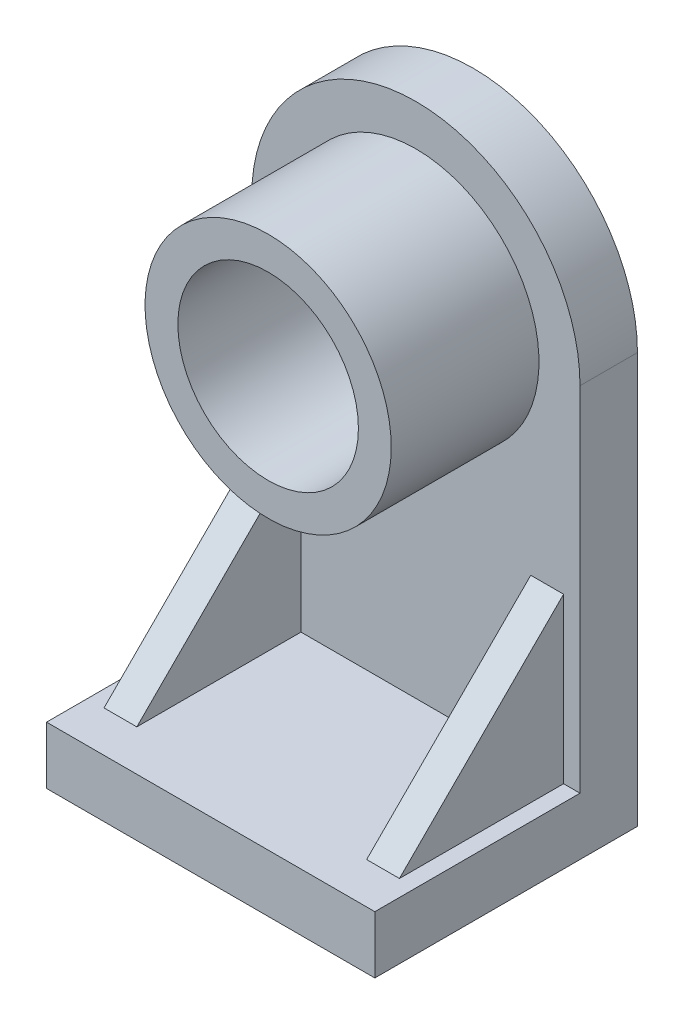
ISO-10303-21;
HEADER;
FILE_DESCRIPTION(('STEP AP214'),'2;1');
FILE_NAME('part.step','',(''),(''),'','','');
FILE_SCHEMA(('AUTOMOTIVE_DESIGN { 1 0 10303 214 1 1 1 1 }'));
ENDSEC;
DATA;
#1=APPLICATION_CONTEXT('core data for automotive mechanical design processes');
#2=APPLICATION_PROTOCOL_DEFINITION('international standard','automotive_design',2000,#1);
#3=PRODUCT_CONTEXT('',#1,'mechanical');
#4=PRODUCT('Part','Part','',(#3));
#5=PRODUCT_RELATED_PRODUCT_CATEGORY('part','',(#4));
#6=PRODUCT_DEFINITION_FORMATION('','',#4);
#7=PRODUCT_DEFINITION_CONTEXT('part definition',#1,'design');
#8=PRODUCT_DEFINITION('design','',#6,#7);
#9=PRODUCT_DEFINITION_SHAPE('','',#8);
#10=(LENGTH_UNIT() NAMED_UNIT(*) SI_UNIT(.MILLI.,.METRE.));
#11=(NAMED_UNIT(*) PLANE_ANGLE_UNIT() SI_UNIT($,.RADIAN.));
#12=(NAMED_UNIT(*) SI_UNIT($,.STERADIAN.) SOLID_ANGLE_UNIT());
#13=UNCERTAINTY_MEASURE_WITH_UNIT(LENGTH_MEASURE(1.E-05),#10,'distance_accuracy_value','');
#14=(GEOMETRIC_REPRESENTATION_CONTEXT(3) GLOBAL_UNCERTAINTY_ASSIGNED_CONTEXT((#13)) GLOBAL_UNIT_ASSIGNED_CONTEXT((#10,
#11,#12)) REPRESENTATION_CONTEXT('',''));
#15=CARTESIAN_POINT('',(0.,0.,0.));
#16=DIRECTION('',(0.,0.,1.));
#17=DIRECTION('',(1.,0.,0.));
#18=AXIS2_PLACEMENT_3D('',#15,#16,#17);
#19=CARTESIAN_POINT('',(20.,7.,0.));
#20=DIRECTION('',(0.,0.,-1.));
#21=DIRECTION('',(0.,1.,0.));
#22=AXIS2_PLACEMENT_3D('',#19,#20,#21);
#23=PLANE('',#22);
#24=DIRECTION('',(0.,-1.,0.));
#25=VECTOR('',#24,1.);
#26=CARTESIAN_POINT('',(-20.,7.,0.));
#27=LINE('',#26,#25);
#28=CARTESIAN_POINT('',(-20.,7.,0.));
#29=VERTEX_POINT('',#28);
#30=CARTESIAN_POINT('',(-20.,0.,0.));
#31=VERTEX_POINT('',#30);
#32=EDGE_CURVE('E189',#29,#31,#27,.T.);
#33=ORIENTED_EDGE('',*,*,#32,.T.);
#34=DIRECTION('',(-1.,0.,0.));
#35=VECTOR('',#34,1.);
#36=CARTESIAN_POINT('',(20.,0.,0.));
#37=LINE('',#36,#35);
#38=CARTESIAN_POINT('',(20.,0.,0.));
#39=VERTEX_POINT('',#38);
#40=EDGE_CURVE('E48',#39,#31,#37,.T.);
#41=ORIENTED_EDGE('',*,*,#40,.F.);
#42=DIRECTION('',(0.,-1.,0.));
#43=VECTOR('',#42,1.);
#44=CARTESIAN_POINT('',(20.,7.,0.));
#45=LINE('',#44,#43);
#46=CARTESIAN_POINT('',(20.,7.,0.));
#47=VERTEX_POINT('',#46);
#48=EDGE_CURVE('E195',#47,#39,#45,.T.);
#49=ORIENTED_EDGE('',*,*,#48,.F.);
#50=DIRECTION('',(-1.,0.,0.));
#51=VECTOR('',#50,1.);
#52=CARTESIAN_POINT('',(20.,7.,0.));
#53=LINE('',#52,#51);
#54=EDGE_CURVE('E206',#47,#29,#53,.T.);
#55=ORIENTED_EDGE('',*,*,#54,.T.);
#56=EDGE_LOOP('',(#33,#41,#49,#55));
#57=FACE_BOUND('',#56,.T.);
#58=ADVANCED_FACE('F41',(#57),#23,.F.);
#59=CARTESIAN_POINT('',(20.,0.,0.));
#60=DIRECTION('',(0.,1.,0.));
#61=DIRECTION('',(0.,0.,1.));
#62=AXIS2_PLACEMENT_3D('',#59,#60,#61);
#63=PLANE('',#62);
#64=DIRECTION('',(0.,0.,-1.));
#65=VECTOR('',#64,1.);
#66=CARTESIAN_POINT('',(-20.,0.,0.));
#67=LINE('',#66,#65);
#68=CARTESIAN_POINT('',(-20.,0.,-32.));
#69=VERTEX_POINT('',#68);
#70=EDGE_CURVE('E207',#31,#69,#67,.T.);
#71=ORIENTED_EDGE('',*,*,#70,.T.);
#72=DIRECTION('',(-1.,0.,0.));
#73=VECTOR('',#72,1.);
#74=CARTESIAN_POINT('',(20.,0.,-32.));
#75=LINE('',#74,#73);
#76=CARTESIAN_POINT('',(20.,0.,-32.));
#77=VERTEX_POINT('',#76);
#78=EDGE_CURVE('E224',#77,#69,#75,.T.);
#79=ORIENTED_EDGE('',*,*,#78,.F.);
#80=DIRECTION('',(0.,0.,-1.));
#81=VECTOR('',#80,1.);
#82=CARTESIAN_POINT('',(20.,0.,0.));
#83=LINE('',#82,#81);
#84=EDGE_CURVE('E194',#39,#77,#83,.T.);
#85=ORIENTED_EDGE('',*,*,#84,.F.);
#86=ORIENTED_EDGE('',*,*,#40,.T.);
#87=EDGE_LOOP('',(#71,#79,#85,#86));
#88=FACE_BOUND('',#87,.T.);
#89=ADVANCED_FACE('F226',(#88),#63,.F.);
#90=CARTESIAN_POINT('',(20.,0.,-32.));
#91=DIRECTION('',(0.,0.,1.));
#92=DIRECTION('',(0.,-1.,0.));
#93=AXIS2_PLACEMENT_3D('',#90,#91,#92);
#94=PLANE('',#93);
#95=DIRECTION('',(0.,1.,0.));
#96=VECTOR('',#95,1.);
#97=CARTESIAN_POINT('',(-20.,0.,-32.));
#98=LINE('',#97,#96);
#99=CARTESIAN_POINT('',(-20.,50.,-32.));
#100=VERTEX_POINT('',#99);
#101=EDGE_CURVE('E211',#69,#100,#98,.T.);
#102=ORIENTED_EDGE('',*,*,#101,.T.);
#103=CARTESIAN_POINT('',(0.,50.,-32.));
#104=DIRECTION('',(0.,0.,1.));
#105=DIRECTION('',(1.,0.,0.));
#106=AXIS2_PLACEMENT_3D('',#103,#104,#105);
#107=CIRCLE('',#106,20.);
#108=CARTESIAN_POINT('',(20.,50.,-32.));
#109=VERTEX_POINT('',#108);
#110=EDGE_CURVE('E188',#100,#109,#107,.F.);
#111=ORIENTED_EDGE('',*,*,#110,.T.);
#112=DIRECTION('',(0.,1.,0.));
#113=VECTOR('',#112,1.);
#114=CARTESIAN_POINT('',(20.,0.,-32.));
#115=LINE('',#114,#113);
#116=EDGE_CURVE('E196',#77,#109,#115,.T.);
#117=ORIENTED_EDGE('',*,*,#116,.F.);
#118=ORIENTED_EDGE('',*,*,#78,.T.);
#119=EDGE_LOOP('',(#102,#111,#117,#118));
#120=FACE_BOUND('',#119,.T.);
#121=ADVANCED_FACE('F243',(#120),#94,.F.);
#122=CARTESIAN_POINT('',(20.,50.,-25.));
#123=DIRECTION('',(0.,0.,-1.));
#124=DIRECTION('',(0.,1.,0.));
#125=AXIS2_PLACEMENT_3D('',#122,#123,#124);
#126=PLANE('',#125);
#127=CARTESIAN_POINT('',(0.,50.,-25.));
#128=DIRECTION('',(0.,0.,-1.));
#129=DIRECTION('',(0.,1.,0.));
#130=AXIS2_PLACEMENT_3D('',#127,#128,#129);
#131=CIRCLE('',#130,15.);
#132=CARTESIAN_POINT('',(0.,65.,-25.));
#133=VERTEX_POINT('',#132);
#134=EDGE_CURVE('E11',#133,#133,#131,.F.);
#135=ORIENTED_EDGE('',*,*,#134,.F.);
#136=EDGE_LOOP('',(#135));
#137=FACE_BOUND('',#136,.T.);
#138=DIRECTION('',(-1.,0.,0.));
#139=VECTOR('',#138,1.);
#140=CARTESIAN_POINT('',(20.,7.00000000000001,-25.));
#141=LINE('',#140,#139);
#142=CARTESIAN_POINT('',(-18.,7.00000000000001,-25.));
#143=VERTEX_POINT('',#142);
#144=CARTESIAN_POINT('',(-20.,7.00000000000001,-25.));
#145=VERTEX_POINT('',#144);
#146=EDGE_CURVE('E140',#143,#145,#141,.T.);
#147=ORIENTED_EDGE('',*,*,#146,.F.);
#148=DIRECTION('',(0.,1.,0.));
#149=VECTOR('',#148,1.);
#150=CARTESIAN_POINT('',(-18.,27.,-25.));
#151=LINE('',#150,#149);
#152=CARTESIAN_POINT('',(-18.,27.,-25.));
#153=VERTEX_POINT('',#152);
#154=EDGE_CURVE('E54',#143,#153,#151,.T.);
#155=ORIENTED_EDGE('',*,*,#154,.T.);
#156=DIRECTION('',(1.,0.,0.));
#157=VECTOR('',#156,1.);
#158=CARTESIAN_POINT('',(-18.,27.,-25.));
#159=LINE('',#158,#157);
#160=CARTESIAN_POINT('',(-14.,27.,-25.));
#161=VERTEX_POINT('',#160);
#162=EDGE_CURVE('E56',#153,#161,#159,.T.);
#163=ORIENTED_EDGE('',*,*,#162,.T.);
#164=DIRECTION('',(0.,1.,0.));
#165=VECTOR('',#164,1.);
#166=CARTESIAN_POINT('',(-14.,27.,-25.));
#167=LINE('',#166,#165);
#168=CARTESIAN_POINT('',(-14.,7.00000000000001,-25.));
#169=VERTEX_POINT('',#168);
#170=EDGE_CURVE('E139',#169,#161,#167,.T.);
#171=ORIENTED_EDGE('',*,*,#170,.F.);
#172=CARTESIAN_POINT('',(14.,7.00000000000001,-25.));
#173=VERTEX_POINT('',#172);
#174=EDGE_CURVE('E126',#173,#169,#141,.T.);
#175=ORIENTED_EDGE('',*,*,#174,.F.);
#176=DIRECTION('',(0.,1.,0.));
#177=VECTOR('',#176,1.);
#178=CARTESIAN_POINT('',(14.,27.,-25.));
#179=LINE('',#178,#177);
#180=CARTESIAN_POINT('',(14.,27.,-25.));
#181=VERTEX_POINT('',#180);
#182=EDGE_CURVE('E169',#173,#181,#179,.T.);
#183=ORIENTED_EDGE('',*,*,#182,.T.);
#184=DIRECTION('',(-1.,0.,0.));
#185=VECTOR('',#184,1.);
#186=CARTESIAN_POINT('',(18.,27.,-25.));
#187=LINE('',#186,#185);
#188=CARTESIAN_POINT('',(18.,27.,-25.));
#189=VERTEX_POINT('',#188);
#190=EDGE_CURVE('E171',#189,#181,#187,.T.);
#191=ORIENTED_EDGE('',*,*,#190,.F.);
#192=DIRECTION('',(0.,1.,0.));
#193=VECTOR('',#192,1.);
#194=CARTESIAN_POINT('',(18.,27.,-25.));
#195=LINE('',#194,#193);
#196=CARTESIAN_POINT('',(18.,7.00000000000001,-25.));
#197=VERTEX_POINT('',#196);
#198=EDGE_CURVE('E157',#197,#189,#195,.T.);
#199=ORIENTED_EDGE('',*,*,#198,.F.);
#200=CARTESIAN_POINT('',(20.,7.00000000000001,-25.));
#201=VERTEX_POINT('',#200);
#202=EDGE_CURVE('E138',#201,#197,#141,.T.);
#203=ORIENTED_EDGE('',*,*,#202,.F.);
#204=DIRECTION('',(0.,-1.,0.));
#205=VECTOR('',#204,1.);
#206=CARTESIAN_POINT('',(20.,50.,-25.));
#207=LINE('',#206,#205);
#208=CARTESIAN_POINT('',(20.,50.,-25.));
#209=VERTEX_POINT('',#208);
#210=EDGE_CURVE('E205',#209,#201,#207,.T.);
#211=ORIENTED_EDGE('',*,*,#210,.F.);
#212=CARTESIAN_POINT('',(0.,50.,-25.));
#213=DIRECTION('',(0.,0.,1.));
#214=DIRECTION('',(1.,0.,0.));
#215=AXIS2_PLACEMENT_3D('',#212,#213,#214);
#216=CIRCLE('',#215,20.);
#217=CARTESIAN_POINT('',(-20.,50.,-25.));
#218=VERTEX_POINT('',#217);
#219=EDGE_CURVE('E183',#218,#209,#216,.F.);
#220=ORIENTED_EDGE('',*,*,#219,.F.);
#221=DIRECTION('',(0.,-1.,0.));
#222=VECTOR('',#221,1.);
#223=CARTESIAN_POINT('',(-20.,50.,-25.));
#224=LINE('',#223,#222);
#225=EDGE_CURVE('E216',#218,#145,#224,.T.);
#226=ORIENTED_EDGE('',*,*,#225,.T.);
#227=EDGE_LOOP('',(#147,#155,#163,#171,#175,#183,#191,#199,#203,#211,#220,#226));
#228=FACE_BOUND('',#227,.T.);
#229=ADVANCED_FACE('F143',(#137,#228),#126,.F.);
#230=CARTESIAN_POINT('',(20.,7.00000000000001,-25.));
#231=DIRECTION('',(0.,-1.,0.));
#232=DIRECTION('',(0.,0.,-1.));
#233=AXIS2_PLACEMENT_3D('',#230,#231,#232);
#234=PLANE('',#233);
#235=DIRECTION('',(1.,0.,0.));
#236=VECTOR('',#235,1.);
#237=CARTESIAN_POINT('',(-18.,7.00000000000001,-5.00000000000001));
#238=LINE('',#237,#236);
#239=CARTESIAN_POINT('',(-18.,7.,-5.));
#240=VERTEX_POINT('',#239);
#241=CARTESIAN_POINT('',(-14.,7.,-5.00000000000001));
#242=VERTEX_POINT('',#241);
#243=EDGE_CURVE('E152',#240,#242,#238,.T.);
#244=ORIENTED_EDGE('',*,*,#243,.F.);
#245=DIRECTION('',(0.,0.,-1.));
#246=VECTOR('',#245,1.);
#247=CARTESIAN_POINT('',(-18.,7.00000000000001,-25.));
#248=LINE('',#247,#246);
#249=EDGE_CURVE('E145',#240,#143,#248,.T.);
#250=ORIENTED_EDGE('',*,*,#249,.T.);
#251=ORIENTED_EDGE('',*,*,#146,.T.);
#252=DIRECTION('',(0.,0.,1.));
#253=VECTOR('',#252,1.);
#254=CARTESIAN_POINT('',(-20.,7.00000000000001,-25.));
#255=LINE('',#254,#253);
#256=EDGE_CURVE('E198',#145,#29,#255,.T.);
#257=ORIENTED_EDGE('',*,*,#256,.T.);
#258=ORIENTED_EDGE('',*,*,#54,.F.);
#259=DIRECTION('',(0.,0.,1.));
#260=VECTOR('',#259,1.);
#261=CARTESIAN_POINT('',(20.,7.00000000000001,-25.));
#262=LINE('',#261,#260);
#263=EDGE_CURVE('E204',#201,#47,#262,.T.);
#264=ORIENTED_EDGE('',*,*,#263,.F.);
#265=ORIENTED_EDGE('',*,*,#202,.T.);
#266=DIRECTION('',(0.,0.,-1.));
#267=VECTOR('',#266,1.);
#268=CARTESIAN_POINT('',(18.,7.00000000000001,-25.));
#269=LINE('',#268,#267);
#270=CARTESIAN_POINT('',(18.,7.,-5.));
#271=VERTEX_POINT('',#270);
#272=EDGE_CURVE('E156',#271,#197,#269,.T.);
#273=ORIENTED_EDGE('',*,*,#272,.F.);
#274=DIRECTION('',(-1.,0.,0.));
#275=VECTOR('',#274,1.);
#276=CARTESIAN_POINT('',(18.,7.00000000000001,-5.00000000000001));
#277=LINE('',#276,#275);
#278=CARTESIAN_POINT('',(14.,7.00000000000001,-5.00000000000001));
#279=VERTEX_POINT('',#278);
#280=EDGE_CURVE('E167',#271,#279,#277,.T.);
#281=ORIENTED_EDGE('',*,*,#280,.T.);
#282=DIRECTION('',(0.,0.,-1.));
#283=VECTOR('',#282,1.);
#284=CARTESIAN_POINT('',(14.,7.00000000000001,-25.));
#285=LINE('',#284,#283);
#286=EDGE_CURVE('E134',#279,#173,#285,.T.);
#287=ORIENTED_EDGE('',*,*,#286,.T.);
#288=ORIENTED_EDGE('',*,*,#174,.T.);
#289=DIRECTION('',(0.,0.,-1.));
#290=VECTOR('',#289,1.);
#291=CARTESIAN_POINT('',(-14.,7.00000000000001,-25.));
#292=LINE('',#291,#290);
#293=EDGE_CURVE('E133',#242,#169,#292,.T.);
#294=ORIENTED_EDGE('',*,*,#293,.F.);
#295=EDGE_LOOP('',(#244,#250,#251,#257,#258,#264,#265,#273,#281,#287,#288,#294));
#296=FACE_BOUND('',#295,.T.);
#297=ADVANCED_FACE('F129',(#296),#234,.F.);
#298=CARTESIAN_POINT('',(20.,0.,0.));
#299=DIRECTION('',(1.,0.,0.));
#300=DIRECTION('',(0.,0.,-1.));
#301=AXIS2_PLACEMENT_3D('',#298,#299,#300);
#302=PLANE('',#301);
#303=ORIENTED_EDGE('',*,*,#48,.T.);
#304=ORIENTED_EDGE('',*,*,#84,.T.);
#305=ORIENTED_EDGE('',*,*,#116,.T.);
#306=DIRECTION('',(0.,0.,1.));
#307=VECTOR('',#306,1.);
#308=CARTESIAN_POINT('',(20.,50.,-32.));
#309=LINE('',#308,#307);
#310=EDGE_CURVE('E199',#109,#209,#309,.T.);
#311=ORIENTED_EDGE('',*,*,#310,.T.);
#312=ORIENTED_EDGE('',*,*,#210,.T.);
#313=ORIENTED_EDGE('',*,*,#263,.T.);
#314=EDGE_LOOP('',(#303,#304,#305,#311,#312,#313));
#315=FACE_BOUND('',#314,.T.);
#316=ADVANCED_FACE('F242',(#315),#302,.T.);
#317=CARTESIAN_POINT('',(-20.,0.,0.));
#318=DIRECTION('',(1.,0.,0.));
#319=DIRECTION('',(0.,0.,-1.));
#320=AXIS2_PLACEMENT_3D('',#317,#318,#319);
#321=PLANE('',#320);
#322=ORIENTED_EDGE('',*,*,#32,.F.);
#323=ORIENTED_EDGE('',*,*,#256,.F.);
#324=ORIENTED_EDGE('',*,*,#225,.F.);
#325=DIRECTION('',(0.,0.,1.));
#326=VECTOR('',#325,1.);
#327=CARTESIAN_POINT('',(-20.,50.,-32.));
#328=LINE('',#327,#326);
#329=EDGE_CURVE('E213',#100,#218,#328,.T.);
#330=ORIENTED_EDGE('',*,*,#329,.F.);
#331=ORIENTED_EDGE('',*,*,#101,.F.);
#332=ORIENTED_EDGE('',*,*,#70,.F.);
#333=EDGE_LOOP('',(#322,#323,#324,#330,#331,#332));
#334=FACE_BOUND('',#333,.T.);
#335=ADVANCED_FACE('F237',(#334),#321,.F.);
#336=CARTESIAN_POINT('',(0.,50.,-32.));
#337=DIRECTION('',(0.,0.,1.));
#338=DIRECTION('',(1.,0.,0.));
#339=AXIS2_PLACEMENT_3D('',#336,#337,#338);
#340=CYLINDRICAL_SURFACE('',#339,20.);
#341=ORIENTED_EDGE('',*,*,#219,.T.);
#342=ORIENTED_EDGE('',*,*,#310,.F.);
#343=ORIENTED_EDGE('',*,*,#110,.F.);
#344=ORIENTED_EDGE('',*,*,#329,.T.);
#345=EDGE_LOOP('',(#341,#342,#343,#344));
#346=FACE_BOUND('',#345,.T.);
#347=ADVANCED_FACE('F252',(#346),#340,.T.);
#348=CARTESIAN_POINT('',(0.,50.,-7.00000000000001));
#349=DIRECTION('',(0.,0.,1.));
#350=DIRECTION('',(1.,0.,0.));
#351=AXIS2_PLACEMENT_3D('',#348,#349,#350);
#352=PLANE('',#351);
#353=CARTESIAN_POINT('',(0.,50.,-7.00000000000001));
#354=DIRECTION('',(0.,0.,1.));
#355=DIRECTION('',(1.,0.,0.));
#356=AXIS2_PLACEMENT_3D('',#353,#354,#355);
#357=CIRCLE('',#356,15.);
#358=CARTESIAN_POINT('',(15.,50.,-7.00000000000001));
#359=VERTEX_POINT('',#358);
#360=EDGE_CURVE('E179',#359,#359,#357,.T.);
#361=ORIENTED_EDGE('',*,*,#360,.T.);
#362=EDGE_LOOP('',(#361));
#363=FACE_BOUND('',#362,.T.);
#364=CARTESIAN_POINT('',(0.,50.,-7.00000000000001));
#365=DIRECTION('',(0.,0.,1.));
#366=DIRECTION('',(1.,0.,0.));
#367=AXIS2_PLACEMENT_3D('',#364,#365,#366);
#368=CIRCLE('',#367,11.);
#369=CARTESIAN_POINT('',(11.,50.,-7.00000000000001));
#370=VERTEX_POINT('',#369);
#371=EDGE_CURVE('E180',#370,#370,#368,.T.);
#372=ORIENTED_EDGE('',*,*,#371,.F.);
#373=EDGE_LOOP('',(#372));
#374=FACE_BOUND('',#373,.T.);
#375=ADVANCED_FACE('F255',(#363,#374),#352,.T.);
#376=CARTESIAN_POINT('',(0.,50.,-7.00000000000001));
#377=DIRECTION('',(0.,0.,-1.));
#378=DIRECTION('',(-1.,0.,0.));
#379=AXIS2_PLACEMENT_3D('',#376,#377,#378);
#380=CYLINDRICAL_SURFACE('',#379,15.);
#381=ORIENTED_EDGE('',*,*,#360,.F.);
#382=EDGE_LOOP('',(#381));
#383=FACE_BOUND('',#382,.T.);
#384=ORIENTED_EDGE('',*,*,#134,.T.);
#385=EDGE_LOOP('',(#384));
#386=FACE_BOUND('',#385,.T.);
#387=ADVANCED_FACE('F257',(#383,#386),#380,.T.);
#388=CARTESIAN_POINT('',(0.,50.,-7.00000000000001));
#389=DIRECTION('',(0.,0.,-1.));
#390=DIRECTION('',(-1.,0.,0.));
#391=AXIS2_PLACEMENT_3D('',#388,#389,#390);
#392=CYLINDRICAL_SURFACE('',#391,11.);
#393=ORIENTED_EDGE('',*,*,#371,.T.);
#394=EDGE_LOOP('',(#393));
#395=FACE_BOUND('',#394,.T.);
#396=CARTESIAN_POINT('',(0.,50.,-25.));
#397=DIRECTION('',(0.,0.,1.));
#398=DIRECTION('',(1.,0.,0.));
#399=AXIS2_PLACEMENT_3D('',#396,#397,#398);
#400=CIRCLE('',#399,11.);
#401=CARTESIAN_POINT('',(11.,50.,-25.));
#402=VERTEX_POINT('',#401);
#403=EDGE_CURVE('E178',#402,#402,#400,.T.);
#404=ORIENTED_EDGE('',*,*,#403,.F.);
#405=EDGE_LOOP('',(#404));
#406=FACE_BOUND('',#405,.T.);
#407=ADVANCED_FACE('F321',(#395,#406),#392,.F.);
#408=ORIENTED_EDGE('',*,*,#403,.T.);
#409=EDGE_LOOP('',(#408));
#410=FACE_BOUND('',#409,.T.);
#411=ADVANCED_FACE('F279',(#410),#126,.F.);
#412=CARTESIAN_POINT('',(18.,7.00000000000001,-5.00000000000001));
#413=DIRECTION('',(0.,-0.707106781186547,-0.707106781186548));
#414=DIRECTION('',(0.,0.707106781186548,-0.707106781186547));
#415=AXIS2_PLACEMENT_3D('',#412,#413,#414);
#416=PLANE('',#415);
#417=DIRECTION('',(0.,-0.707106781186548,0.707106781186547));
#418=VECTOR('',#417,1.);
#419=CARTESIAN_POINT('',(14.,7.00000000000001,-5.00000000000001));
#420=LINE('',#419,#418);
#421=EDGE_CURVE('E159',#181,#279,#420,.T.);
#422=ORIENTED_EDGE('',*,*,#421,.T.);
#423=ORIENTED_EDGE('',*,*,#280,.F.);
#424=DIRECTION('',(0.,-0.707106781186548,0.707106781186547));
#425=VECTOR('',#424,1.);
#426=CARTESIAN_POINT('',(18.,7.00000000000001,-5.00000000000001));
#427=LINE('',#426,#425);
#428=EDGE_CURVE('E162',#189,#271,#427,.T.);
#429=ORIENTED_EDGE('',*,*,#428,.F.);
#430=ORIENTED_EDGE('',*,*,#190,.T.);
#431=EDGE_LOOP('',(#422,#423,#429,#430));
#432=FACE_BOUND('',#431,.T.);
#433=ADVANCED_FACE('F319',(#432),#416,.F.);
#434=CARTESIAN_POINT('',(18.,0.,0.));
#435=DIRECTION('',(1.,0.,0.));
#436=DIRECTION('',(0.,0.,-1.));
#437=AXIS2_PLACEMENT_3D('',#434,#435,#436);
#438=PLANE('',#437);
#439=ORIENTED_EDGE('',*,*,#272,.T.);
#440=ORIENTED_EDGE('',*,*,#198,.T.);
#441=ORIENTED_EDGE('',*,*,#428,.T.);
#442=EDGE_LOOP('',(#439,#440,#441));
#443=FACE_BOUND('',#442,.T.);
#444=ADVANCED_FACE('F352',(#443),#438,.T.);
#445=CARTESIAN_POINT('',(14.,0.,0.));
#446=DIRECTION('',(1.,0.,0.));
#447=DIRECTION('',(0.,0.,-1.));
#448=AXIS2_PLACEMENT_3D('',#445,#446,#447);
#449=PLANE('',#448);
#450=ORIENTED_EDGE('',*,*,#286,.F.);
#451=ORIENTED_EDGE('',*,*,#421,.F.);
#452=ORIENTED_EDGE('',*,*,#182,.F.);
#453=EDGE_LOOP('',(#450,#451,#452));
#454=FACE_BOUND('',#453,.T.);
#455=ADVANCED_FACE('F364',(#454),#449,.F.);
#456=CARTESIAN_POINT('',(-18.,7.00000000000001,-5.00000000000001));
#457=DIRECTION('',(0.,0.707106781186547,0.707106781186548));
#458=DIRECTION('',(0.,-0.707106781186548,0.707106781186547));
#459=AXIS2_PLACEMENT_3D('',#456,#457,#458);
#460=PLANE('',#459);
#461=DIRECTION('',(0.,-0.707106781186548,0.707106781186547));
#462=VECTOR('',#461,1.);
#463=CARTESIAN_POINT('',(-14.,7.00000000000001,-5.00000000000001));
#464=LINE('',#463,#462);
#465=EDGE_CURVE('E144',#161,#242,#464,.T.);
#466=ORIENTED_EDGE('',*,*,#465,.F.);
#467=ORIENTED_EDGE('',*,*,#162,.F.);
#468=DIRECTION('',(0.,-0.707106781186548,0.707106781186547));
#469=VECTOR('',#468,1.);
#470=CARTESIAN_POINT('',(-18.,7.00000000000001,-5.00000000000001));
#471=LINE('',#470,#469);
#472=EDGE_CURVE('E410',#153,#240,#471,.T.);
#473=ORIENTED_EDGE('',*,*,#472,.T.);
#474=ORIENTED_EDGE('',*,*,#243,.T.);
#475=EDGE_LOOP('',(#466,#467,#473,#474));
#476=FACE_BOUND('',#475,.T.);
#477=ADVANCED_FACE('F372',(#476),#460,.T.);
#478=CARTESIAN_POINT('',(-18.,0.,0.));
#479=DIRECTION('',(-1.,0.,0.));
#480=DIRECTION('',(0.,0.,-1.));
#481=AXIS2_PLACEMENT_3D('',#478,#479,#480);
#482=PLANE('',#481);
#483=ORIENTED_EDGE('',*,*,#249,.F.);
#484=ORIENTED_EDGE('',*,*,#472,.F.);
#485=ORIENTED_EDGE('',*,*,#154,.F.);
#486=EDGE_LOOP('',(#483,#484,#485));
#487=FACE_BOUND('',#486,.T.);
#488=ADVANCED_FACE('F383',(#487),#482,.T.);
#489=CARTESIAN_POINT('',(-14.,0.,0.));
#490=DIRECTION('',(-1.,0.,0.));
#491=DIRECTION('',(0.,0.,-1.));
#492=AXIS2_PLACEMENT_3D('',#489,#490,#491);
#493=PLANE('',#492);
#494=ORIENTED_EDGE('',*,*,#293,.T.);
#495=ORIENTED_EDGE('',*,*,#170,.T.);
#496=ORIENTED_EDGE('',*,*,#465,.T.);
#497=EDGE_LOOP('',(#494,#495,#496));
#498=FACE_BOUND('',#497,.T.);
#499=ADVANCED_FACE('F150',(#498),#493,.F.);
#500=CLOSED_SHELL('',(#58,#89,#121,#229,#297,#316,#335,#347,#375,#387,#407,#411,#433,#444,#455,
#477,#488,#499));
#501=MANIFOLD_SOLID_BREP('B2',#500);
#502=ADVANCED_BREP_SHAPE_REPRESENTATION('',(#18,#501),#14);
#503=SHAPE_DEFINITION_REPRESENTATION(#9,#502);
ENDSEC;
END-ISO-10303-21;
